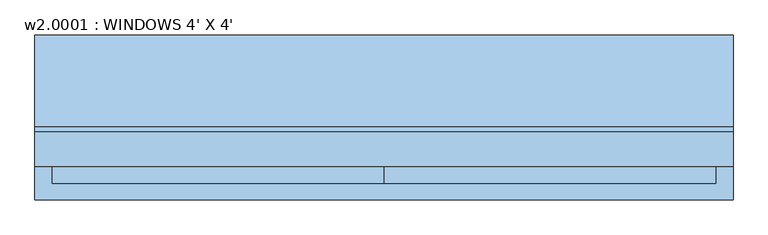
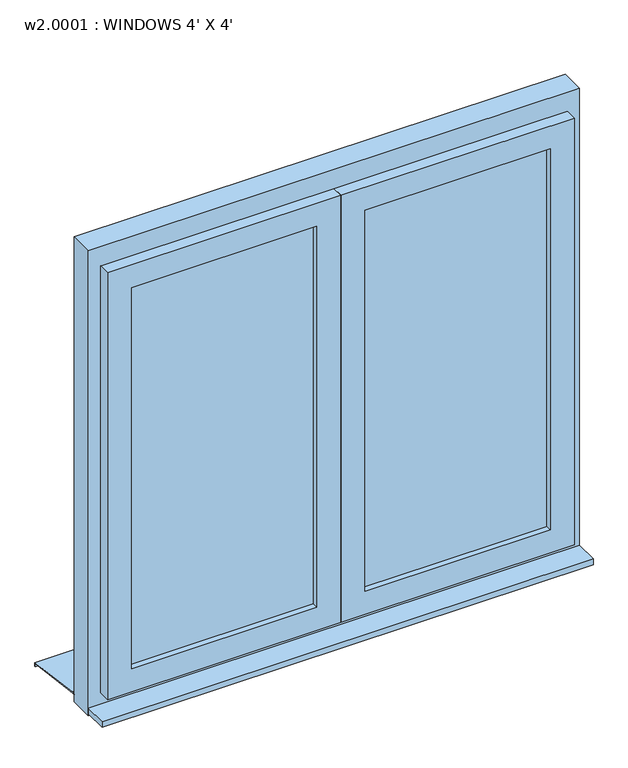
"""IFC4 building model written with IfcOpenShell, lengths in millimetres: window geometry, w2.0001 : WINDOWS 4' X 4'."""

from ifc_helpers import new_model, si_unit, frame, origin, place, context, project, spatial, polyline, outline, extrude, faceted_brep, source, transform, mapped, element, save


def w2_0001_windows_4_x_4_9dec5fc7(model_context):
    return source(origin(), model_context, "Body", "SolidModel", [
        extrude(outline(polyline([(-15.6778457, 1020.0), (144.3, 1000.0), (144.3, 990.0), (142.3, 990.0), (142.3, 998.3604634), (-15.8759277, 1018.0), (-25.7, 1018.0), (-25.7, 1020.0), (-15.6778457, 1020.0)])), frame((-609.6, 0.0, 0.0), z_axis=(1.0, 0.0, 0.0), x_axis=(0.0, 1.0, 0.0)), (0.0, 0.0, 1.0), 1219.2),
        extrude(outline(polyline([(-609.6, -144.3), (-609.6, -85.7), (609.6, -85.7), (609.6, -144.3), (-609.6, -144.3)])), frame((0.0, 0.0, 1005.0), z_axis=(0.0, 0.0, 1.0), x_axis=(1.0, 0.0, 0.0)), (0.0, 0.0, 1.0), 15.0),
        extrude(outline(polyline([(60.0, -70.7), (519.6, -70.7), (519.6, -100.7), (60.0, -100.7), (60.0, -70.7)])), frame((0.0, 0.0, 1110.0), z_axis=(0.0, 0.0, 1.0), x_axis=(1.0, 0.0, 0.0)), (0.0, 0.0, 1.0), 999.2),
        extrude(outline(polyline([(-519.6, -70.7), (-60.0, -70.7), (-60.0, -100.7), (-519.6, -100.7), (-519.6, -70.7)])), frame((0.0, 0.0, 1110.0), z_axis=(0.0, 0.0, 1.0), x_axis=(1.0, 0.0, 0.0)), (0.0, 0.0, 1.0), 999.2),
        extrude(outline(polyline([(2219.2, -609.6), (1000.0, -609.6), (1000.0, 609.6), (2219.2, 609.6), (2219.2, -609.6)]), holes=[polyline([(2139.2, -549.6), (2139.2, 549.6), (1080.0, 549.6), (1080.0, -549.6), (2139.2, -549.6)])]), frame((0.0, -85.7, 0.0), z_axis=(0.0, 1.0, 0.0), x_axis=(0.0, 0.0, 1.0)), (0.0, 0.0, 1.0), 60.0),
        extrude(outline(polyline([(30.0, -85.7), (-30.0, -85.7), (-30.0, -25.7), (30.0, -25.7), (30.0, -85.7)])), frame((0.0, 0.0, 1080.0), z_axis=(0.0, 0.0, 1.0), x_axis=(1.0, 0.0, 0.0)), (0.0, 0.0, 1.0), 1059.2),
        faceted_brep([(30.0, -85.7, 1080.0), (30.0, -55.7, 1080.0), (549.6, -55.7, 1080.0), (549.6, -85.7, 1080.0), (549.6, -55.7, 2139.2), (549.6, -85.7, 2139.2), (30.0, -55.7, 2139.2), (519.6, -55.7, 2109.2), (60.0, -55.7, 2109.2), (60.0, -55.7, 1110.0), (519.6, -55.7, 1110.0), (579.6, -85.7, 1050.0), (0.0, -85.7, 1050.0), (0.0, -85.7, 2169.2), (579.6, -85.7, 2169.2), (30.0, -85.7, 2139.2), (0.0, -115.7, 1050.0), (579.6, -115.7, 1050.0), (579.6, -115.7, 2169.2), (0.0, -115.7, 2169.2), (519.6, -115.7, 1110.0), (60.0, -115.7, 1110.0), (60.0, -115.7, 2109.2), (519.6, -115.7, 2109.2)], [[[0, 1, 2, 3]], [[3, 2, 4, 5]], [[2, 1, 6, 4], [7, 8, 9, 10]], [[11, 12, 13, 14], [5, 15, 0, 3]], [[16, 12, 11, 17]], [[17, 11, 14, 18]], [[18, 19, 16, 17], [20, 21, 22, 23]], [[9, 21, 20, 10]], [[10, 20, 23, 7]], [[15, 6, 1, 0]], [[19, 13, 12, 16]], [[8, 22, 21, 9]], [[5, 4, 6, 15]], [[18, 14, 13, 19]], [[7, 23, 22, 8]]]),
        faceted_brep([(-549.6, -85.7, 1080.0), (-549.6, -55.7, 1080.0), (-30.0, -55.7, 1080.0), (-30.0, -85.7, 1080.0), (-30.0, -55.7, 2139.2), (-30.0, -85.7, 2139.2), (-549.6, -55.7, 2139.2), (-60.0, -55.7, 2109.2), (-519.6, -55.7, 2109.2), (-519.6, -55.7, 1110.0), (-60.0, -55.7, 1110.0), (0.0, -85.7, 1050.0), (-579.6, -85.7, 1050.0), (-579.6, -85.7, 2169.2), (0.0, -85.7, 2169.2), (-549.6, -85.7, 2139.2), (-579.6, -115.7, 1050.0), (0.0, -115.7, 1050.0), (0.0, -115.7, 2169.2), (-579.6, -115.7, 2169.2), (-60.0, -115.7, 1110.0), (-519.6, -115.7, 1110.0), (-519.6, -115.7, 2109.2), (-60.0, -115.7, 2109.2)], [[[0, 1, 2, 3]], [[3, 2, 4, 5]], [[2, 1, 6, 4], [7, 8, 9, 10]], [[11, 12, 13, 14], [5, 15, 0, 3]], [[16, 12, 11, 17]], [[17, 11, 14, 18]], [[18, 19, 16, 17], [20, 21, 22, 23]], [[9, 21, 20, 10]], [[10, 20, 23, 7]], [[15, 6, 1, 0]], [[19, 13, 12, 16]], [[8, 22, 21, 9]], [[5, 4, 6, 15]], [[18, 14, 13, 19]], [[7, 23, 22, 8]]]),
    ])


if __name__ == "__main__":
    model = new_model("IFC4")
    model_context = context("Model", 3, world=origin())
    ifc_project = project(units=[si_unit("LENGTHUNIT", "METRE", prefix="MILLI")], contexts=[model_context])
    site = spatial("IfcSite", under=ifc_project)
    building = spatial("IfcBuilding", under=site)
    placement = place(None, origin())
    w2_0001_windows_4_x_4_shape = w2_0001_windows_4_x_4_9dec5fc7(model_context)
    element("IfcWindow", 1, ObjectType="w2.0001 : WINDOWS 4' X 4'", at=placement, inside=building, context=model_context, shape_type="MappedRepresentation", body=[
        mapped(w2_0001_windows_4_x_4_shape, transform((0.0, 0.0, 0.0), x_axis=(1.0, 0.0, 0.0), y_axis=(0.0, 1.0, 0.0), z_axis=(0.0, 0.0, 1.0))),
    ])
    save(model, "model.ifc")

# Revit data of these elements
# Type "w2.0001 : WINDOWS 4' X 4'"
#   Type Mark = "21"
#   Operation = "DoublePanelVertical"
#   Keynote = "16.05.01"
#   Analytic Construction = "<None>"
#   Rough Width = 4' - 0"
#   Rough Height = 4' - 0"
#   Rahmentiefe = 0' - 2.3622"
#   Rahmenhöhe unten = 0' - 3.14961"
#   Rahmehöhe oben = 0' - 3.14961"
#   Rahmenbreite = 0' - 2.3622"
#   Height = 4' - 0"
#   Flügeltiefe = 0' - 2.3622"
#   Flügelbreite = 0' - 2.3622"
#   Einbautiefe (von außen) [instance default] = 0' - 5.51181"
#   Width = 4' - 0"
#   Kippflügel [instance default] = yes
#   Drehflügel im Grundriß darstellen [instance default] = no
#   Drehflügel [instance default] = yes
#   Define Thermal Properties by = 1
#   Rahmen [instance default] = none
#   Glas [instance default] = none
#   Flügel [instance default] = none
#   Fensterbank aussen [instance default] = none
#   Fensterbank innen [instance default] = none
#   Wall Closure = (empty or 0)
# Element 1 (IfcWindow, "w2.0001 : WINDOWS 4' X 4'")
#   Materials on its faces: "Fenster - Kunststoff", "Fenster - Kunststoff weiss", "Glass", "Fenster - Holz"
# Materials
#   "Fenster - Kunststoff": colour RGB 249 249 249, transparency 0
#   "Fenster - Kunststoff weiss": colour RGB 249 249 249, transparency 0
#   "Glass": class "Glass", colour RGB 0 128 192, transparency 0.75, Description = "Soda Lime Glass", Cost = 0
#   "Fenster - Holz": colour RGB 216 135 75, transparency 0
